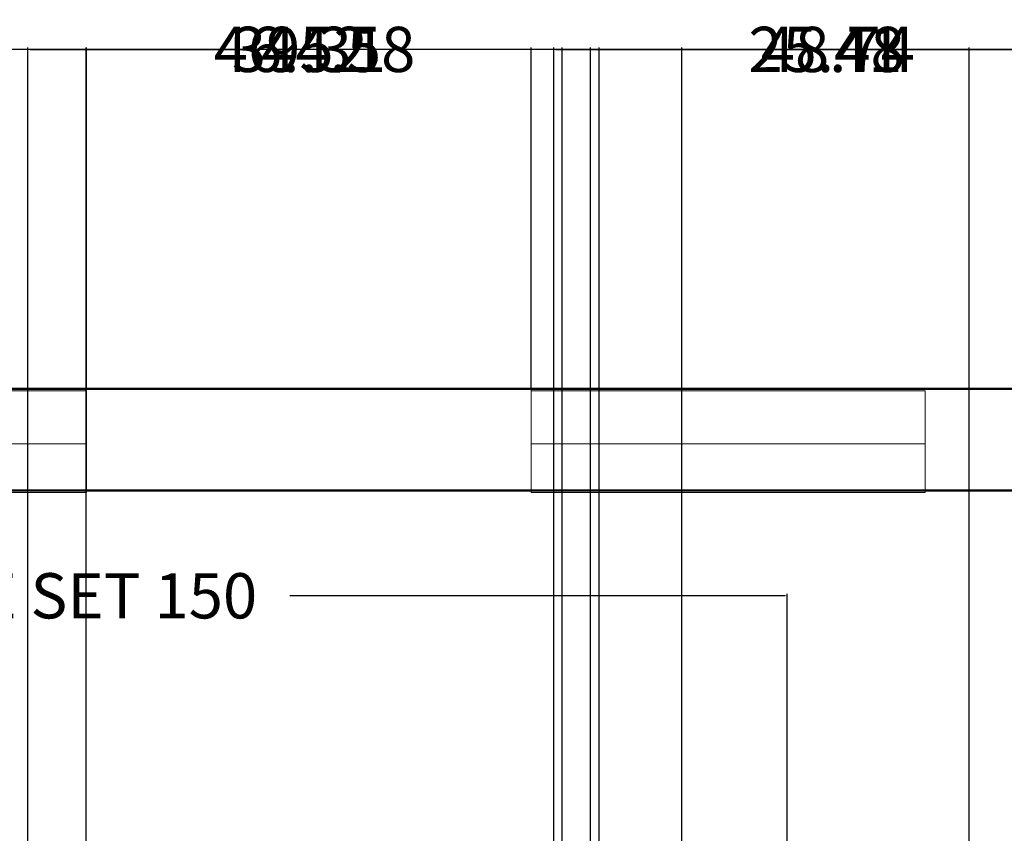
# Model space of a CAD drawing. Units: inches. Extents: x 1454 to 2136, y 626 to 1213.
# Tile 18 of 23: x 1654 to 1741, y 1141 to 1213. Entities that reach past the tile are written whole.
import ezdxf

# ---------------------------------------------------------------- set-up
doc = ezdxf.new("R2010")
doc.units = ezdxf.units.IN
doc.header["$MEASUREMENT"] = 0
for name, color, linetype, lineweight in [('A-ANNO-DIMS', 2, 'Continuous', 18), ('A-GLAZ', 4, 'Continuous', 18), ('A-WALL', 7, 'Continuous', 50)]:
    doc.layers.add(name, color=color, linetype=linetype, lineweight=lineweight)
doc.styles.get("Standard").update_dxf_attribs({"font": 'arial.ttf'})
doc.dimstyles.get("Standard").update_dxf_attribs({"dimtxt": 4, "dimasz": 0.18, "dimexe": 0.18, "dimexo": 0.0625, "dimgap": 0.09, "dimtad": 0, "dimtih": 1, "dimtoh": 1, "dimdec": 0, "dimrnd": 6, "dimzin": 0, "dimdsep": 46, "dimlunit": 3, "dimtxsty": 'Standard', "dimcen": 0.09, "dimadec": 0, "dimazin": 0, "dimtfac": 1, "dimtdec": 0, "dimtofl": 0, "dimtmove": 0, "dimatfit": 3, "dimfxl": 1, "dimtolj": 1, "dimtzin": 0, "dimarcsym": 0})

# ---------------------------------------------------------------- blocks, each defined once
blk = doc.blocks.new('WIN-34_84')
blk.add_line((34.84, 4.305), (0, 4.305))
blk.add_lwpolyline([(34.84, 0), (0, 0), (0, 9), (34.84, 9)], close=True)
blk = doc.blocks.new('*D23')
at = {"layer": 'A-ANNO-DIMS', "color": 0, "lineweight": -2, "transparency": 16777216}
for p, q in [((1571.674, 1139.532), (1571.674, 1162.157)), ((1571.854, 1161.977), (1615.675, 1161.977)), ((1721.545, 1161.977), (1677.724, 1161.977)), ((1721.725, 1139.532), (1721.725, 1162.157))]:
    blk.add_line(p, q, dxfattribs=at)
at = {"layer": 'A-ANNO-DIMS', "color": 0, "transparency": 16777216}
for points in [[(1571.854, 1162.007), (1571.854, 1161.947), (1571.674, 1161.977)], [(1721.545, 1162.007), (1721.545, 1161.947), (1721.725, 1161.977)]]:
    blk.add_solid(points, dxfattribs=at)
at = {"layer": 'Defpoints', "color": 0, "transparency": 16777216}
for p in [(1721.725, 1161.977), (1571.674, 1139.469), (1721.725, 1139.469)]:
    blk.add_point(p, dxfattribs=at)
at = {"layer": 'A-ANNO-DIMS', "color": 0, "transparency": 16777216, "insert": (1646.7, 1161.977), "char_height": 4, "attachment_point": 5}
blk.add_mtext('\\A1;CONFERENCE SET 150', dxfattribs=at)
blk = doc.blocks.new('*D29')
at = {"layer": 'A-ANNO-DIMS', "color": 0, "lineweight": -2, "transparency": 16777216}
for p, q in [((1546.556, 1171.345), (1546.556, 1210.464)), ((1750.556, 1171.345), (1750.556, 1210.464)), ((1546.736, 1210.284), (1644.022, 1210.284)), ((1750.376, 1210.284), (1653.091, 1210.284))]:
    blk.add_line(p, q, dxfattribs=at)
at = {"layer": 'A-ANNO-DIMS', "color": 0, "transparency": 16777216}
for points in [[(1546.736, 1210.314), (1546.736, 1210.254), (1546.556, 1210.284)], [(1750.376, 1210.314), (1750.376, 1210.254), (1750.556, 1210.284)]]:
    blk.add_solid(points, dxfattribs=at)
at = {"layer": 'Defpoints', "color": 0, "transparency": 16777216}
for p in [(1750.556, 1210.284), (1546.556, 1171.282), (1750.556, 1171.282)]:
    blk.add_point(p, dxfattribs=at)
at = {"layer": 'A-ANNO-DIMS', "color": 0, "transparency": 16777216, "insert": (1648.556, 1210.284), "char_height": 4, "attachment_point": 5}
blk.add_mtext('\\A1;204', dxfattribs=at)
blk = doc.blocks.new('*D44')
at = {"layer": 'A-ANNO-DIMS', "color": 0, "lineweight": -2, "transparency": 16777216}
for p, q in [((1701.076, 909.11), (1701.076, 1210.464)), ((1885.25, 909.11), (1885.25, 1210.464)), ((1701.256, 1210.284), (1784.958, 1210.284)), ((1885.07, 1210.284), (1801.368, 1210.284))]:
    blk.add_line(p, q, dxfattribs=at)
at = {"layer": 'A-ANNO-DIMS', "color": 0, "transparency": 16777216}
for points in [[(1701.256, 1210.314), (1701.256, 1210.254), (1701.076, 1210.284)], [(1885.07, 1210.314), (1885.07, 1210.254), (1885.25, 1210.284)]]:
    blk.add_solid(points, dxfattribs=at)
at = {"layer": 'Defpoints', "color": 0, "transparency": 16777216}
for p in [(1885.25, 1210.284), (1701.076, 909.048), (1885.25, 909.048)]:
    blk.add_point(p, dxfattribs=at)
at = {"layer": 'A-ANNO-DIMS', "color": 0, "transparency": 16777216, "insert": (1793.163, 1210.284), "char_height": 4, "attachment_point": 5}
blk.add_mtext('\\A1;184.17', dxfattribs=at)
blk = doc.blocks.new('*D45')
at = {"layer": 'A-ANNO-DIMS', "color": 0, "lineweight": -2, "transparency": 16777216}
for p, q in [((1654.556, 913.345), (1654.556, 1210.464)), ((1701.076, 909.11), (1701.076, 1210.464)), ((1654.736, 1210.284), (1670.917, 1210.284)), ((1700.896, 1210.284), (1684.715, 1210.284))]:
    blk.add_line(p, q, dxfattribs=at)
at = {"layer": 'A-ANNO-DIMS', "color": 0, "transparency": 16777216}
for points in [[(1654.736, 1210.314), (1654.736, 1210.254), (1654.556, 1210.284)], [(1700.896, 1210.314), (1700.896, 1210.254), (1701.076, 1210.284)]]:
    blk.add_solid(points, dxfattribs=at)
at = {"layer": 'Defpoints', "color": 0, "transparency": 16777216}
for p in [(1701.076, 1210.284), (1654.556, 913.282), (1701.076, 909.048)]:
    blk.add_point(p, dxfattribs=at)
at = {"layer": 'A-ANNO-DIMS', "color": 0, "transparency": 16777216, "insert": (1677.816, 1210.284), "char_height": 4, "attachment_point": 5}
blk.add_mtext('\\A1;46.52', dxfattribs=at)
blk = doc.blocks.new('*D51')
at = {"layer": 'A-ANNO-DIMS', "color": 0, "lineweight": -2, "transparency": 16777216}
for p, q in [((1659.76, 1180.166), (1659.76, 1210.464)), ((1699.073, 1180.166), (1699.073, 1210.464)), ((1659.94, 1210.284), (1672.965, 1210.284)), ((1698.893, 1210.284), (1685.868, 1210.284))]:
    blk.add_line(p, q, dxfattribs=at)
at = {"layer": 'A-ANNO-DIMS', "color": 0, "transparency": 16777216}
for points in [[(1659.94, 1210.314), (1659.94, 1210.254), (1659.76, 1210.284)], [(1698.893, 1210.314), (1698.893, 1210.254), (1699.073, 1210.284)]]:
    blk.add_solid(points, dxfattribs=at)
at = {"layer": 'Defpoints', "color": 0, "transparency": 16777216}
for p in [(1699.073, 1210.284), (1659.76, 1180.104), (1699.073, 1180.104)]:
    blk.add_point(p, dxfattribs=at)
at = {"layer": 'A-ANNO-DIMS', "color": 0, "transparency": 16777216, "insert": (1679.416, 1210.284), "char_height": 4, "attachment_point": 5}
blk.add_mtext('\\A1;39.31', dxfattribs=at)
blk = doc.blocks.new('*D68')
at = {"layer": 'A-ANNO-DIMS', "color": 0, "lineweight": -2, "transparency": 16777216}
for p, q in [((1659.724, 1027.329), (1659.724, 1210.464)), ((1704.308, 1027.329), (1704.308, 1210.464)), ((1659.904, 1210.284), (1675.092, 1210.284)), ((1704.128, 1210.284), (1688.939, 1210.284))]:
    blk.add_line(p, q, dxfattribs=at)
at = {"layer": 'A-ANNO-DIMS', "color": 0, "transparency": 16777216}
for points in [[(1659.904, 1210.314), (1659.904, 1210.254), (1659.724, 1210.284)], [(1704.128, 1210.314), (1704.128, 1210.254), (1704.308, 1210.284)]]:
    blk.add_solid(points, dxfattribs=at)
at = {"layer": 'Defpoints', "color": 0, "transparency": 16777216}
for p in [(1704.308, 1210.284), (1659.724, 1027.267), (1704.308, 1027.267)]:
    blk.add_point(p, dxfattribs=at)
at = {"layer": 'A-ANNO-DIMS', "color": 0, "transparency": 16777216, "insert": (1682.016, 1210.284), "char_height": 4, "attachment_point": 5}
blk.add_mtext('\\A1;44.58', dxfattribs=at)
blk = doc.blocks.new('*D71')
at = {"layer": 'A-ANNO-DIMS', "color": 0, "lineweight": -2, "transparency": 16777216}
for p, q in [((1712.389, 694.263), (1712.389, 1210.464)), ((1737.8, 694.263), (1737.8, 1210.464)), ((1712.569, 1210.284), (1718.607, 1210.284)), ((1737.62, 1210.284), (1731.581, 1210.284))]:
    blk.add_line(p, q, dxfattribs=at)
at = {"layer": 'A-ANNO-DIMS', "color": 0, "transparency": 16777216}
for points in [[(1712.569, 1210.314), (1712.569, 1210.254), (1712.389, 1210.284)], [(1737.62, 1210.314), (1737.62, 1210.254), (1737.8, 1210.284)]]:
    blk.add_solid(points, dxfattribs=at)
at = {"layer": 'Defpoints', "color": 0, "transparency": 16777216}
for p in [(1737.8, 1210.284), (1712.389, 694.201), (1737.8, 694.201)]:
    blk.add_point(p, dxfattribs=at)
at = {"layer": 'A-ANNO-DIMS', "color": 0, "transparency": 16777216, "insert": (1725.094, 1210.284), "char_height": 4, "attachment_point": 5}
blk.add_mtext('\\A1;25.41', dxfattribs=at)
blk = doc.blocks.new('*D78')
at = {"layer": 'A-ANNO-DIMS', "color": 0, "lineweight": -2, "transparency": 16777216}
for p, q in [((1705.076, 833.11), (1705.076, 1210.464)), ((1753.076, 833.11), (1753.076, 1210.464)), ((1705.256, 1210.284), (1726.037, 1210.284)), ((1752.896, 1210.284), (1732.116, 1210.284))]:
    blk.add_line(p, q, dxfattribs=at)
at = {"layer": 'A-ANNO-DIMS', "color": 0, "transparency": 16777216}
for points in [[(1705.256, 1210.314), (1705.256, 1210.254), (1705.076, 1210.284)], [(1752.896, 1210.314), (1752.896, 1210.254), (1753.076, 1210.284)]]:
    blk.add_solid(points, dxfattribs=at)
at = {"layer": 'Defpoints', "color": 0, "transparency": 16777216}
for p in [(1753.076, 1210.284), (1705.076, 833.048), (1753.076, 833.048)]:
    blk.add_point(p, dxfattribs=at)
at = {"layer": 'A-ANNO-DIMS', "color": 0, "transparency": 16777216, "insert": (1729.076, 1210.284), "char_height": 4, "attachment_point": 5}
blk.add_mtext('\\A1;48', dxfattribs=at)
blk = doc.blocks.new('*D81')
at = {"layer": 'A-ANNO-DIMS', "color": 0, "lineweight": -2, "transparency": 16777216}
for p, q in [((1701.818, 1088.128), (1701.818, 1210.464)), ((1750.556, 1027.345), (1750.556, 1210.464)), ((1701.998, 1210.284), (1719.276, 1210.284)), ((1750.376, 1210.284), (1733.098, 1210.284))]:
    blk.add_line(p, q, dxfattribs=at)
at = {"layer": 'A-ANNO-DIMS', "color": 0, "transparency": 16777216}
for points in [[(1701.998, 1210.314), (1701.998, 1210.254), (1701.818, 1210.284)], [(1750.376, 1210.314), (1750.376, 1210.254), (1750.556, 1210.284)]]:
    blk.add_solid(points, dxfattribs=at)
at = {"layer": 'Defpoints', "color": 0, "transparency": 16777216}
for p in [(1701.818, 1210.284), (1701.818, 1088.066), (1750.556, 1027.282)]:
    blk.add_point(p, dxfattribs=at)
at = {"layer": 'A-ANNO-DIMS', "color": 0, "transparency": 16777216, "insert": (1726.187, 1210.284), "char_height": 4, "attachment_point": 5}
blk.add_mtext('\\A1;48.74', dxfattribs=at)

msp = doc.modelspace()

# ---------------------------------------------------------------- linework, layer by layer
at = {"layer": 'A-WALL'}
for p, q in [((1759.5563, 1180.2825), (1537.5563, 1180.2825)), ((1750.5563, 1171.2825), (1546.5563, 1171.2825))]:
    msp.add_line(p, q, dxfattribs=at)

# ---------------------------------------------------------------- block references
at = {"layer": 'A-GLAZ'}
for p in [(1624.9195, 1171.1038), (1699.0727, 1171.1038)]:
    msp.add_blockref('WIN-34_84', p, dxfattribs=at)

# ---------------------------------------------------------------- dimensions: what is measured, and where the dimension line sits
at = {"layer": 'A-ANNO-DIMS'}
for base, p1, p2, override, picture, middle in [((1750.5563, 1210.2845), (1546.5563, 1171.2825), (1750.5563, 1171.2825), {"dimdec": 0, "dimlfac": 1, "dimrnd": 0, "dimzin": 0, "dimdsep": 46, "dimlunit": 2}, '*D29', (1648.5563, 1210.2845)), ((1701.0763, 1210.2845), (1654.5563, 913.2825), (1701.0763, 909.0476), {"dimdec": 2, "dimlfac": 1, "dimrnd": 0, "dimzin": 0, "dimdsep": 46, "dimlunit": 2}, '*D45', (1677.8163, 1210.2845)), ((1704.308, 1210.2845), (1659.7237, 1027.2667), (1704.308, 1027.2667), {"dimdec": 2, "dimlfac": 1, "dimrnd": 0, "dimzin": 0, "dimdsep": 46, "dimlunit": 2}, '*D68', (1682.0158, 1210.2845)), ((1699.0727, 1210.2845), (1659.7598, 1180.1038), (1699.0727, 1180.1038), {"dimdec": 2, "dimlfac": 1, "dimrnd": 0, "dimzin": 0, "dimdsep": 46, "dimlunit": 2}, '*D51', (1679.4163, 1210.2845)), ((1885.2497, 1210.2845), (1701.0763, 909.0476), (1885.2497, 909.0476), {"dimdec": 2, "dimlfac": 1, "dimrnd": 0, "dimzin": 0, "dimdsep": 46, "dimlunit": 2}, '*D44', (1793.163, 1210.2845)), ((1701.8177, 1210.2845), (1750.5563, 1027.2825), (1701.8177, 1088.0655), {"dimdec": 2, "dimlfac": 1, "dimrnd": 0, "dimzin": 0, "dimdsep": 46, "dimlunit": 2}, '*D81', (1726.187, 1210.2845)), ((1753.0763, 1210.2845), (1705.0763, 833.0476), (1753.0763, 833.0476), {"dimdec": 0, "dimlfac": 1, "dimrnd": 0, "dimzin": 0, "dimdsep": 46, "dimlunit": 2}, '*D78', (1729.0763, 1210.2845)), ((1737.8001, 1210.2845), (1712.3887, 694.2005), (1737.8001, 694.2005), {"dimdec": 2, "dimlfac": 1, "dimrnd": 0, "dimzin": 0, "dimdsep": 46, "dimlunit": 2}, '*D71', (1725.0944, 1210.2845))]:
    dim = msp.add_linear_dim(base=base, p1=p1, p2=p2, dimstyle='Standard', override=override, dxfattribs=at)
    dim.commit()
    dim.dimension.update_dxf_attribs({"geometry": picture, "text_midpoint": middle})
dim = msp.add_linear_dim(base=(1721.7253, 1161.9768), p1=(1571.674, 1139.4691), p2=(1721.7253, 1139.4691), text='CONFERENCE SET <>', dimstyle='Standard', override={"dimdec": 0, "dimlfac": 1, "dimrnd": 0, "dimzin": 0, "dimdsep": 46, "dimlunit": 2}, dxfattribs=at)
dim.commit()
dim.dimension.update_dxf_attribs({"geometry": '*D23', "text_midpoint": (1646.6996, 1161.9768)})

doc.saveas('drawing.dxf')
